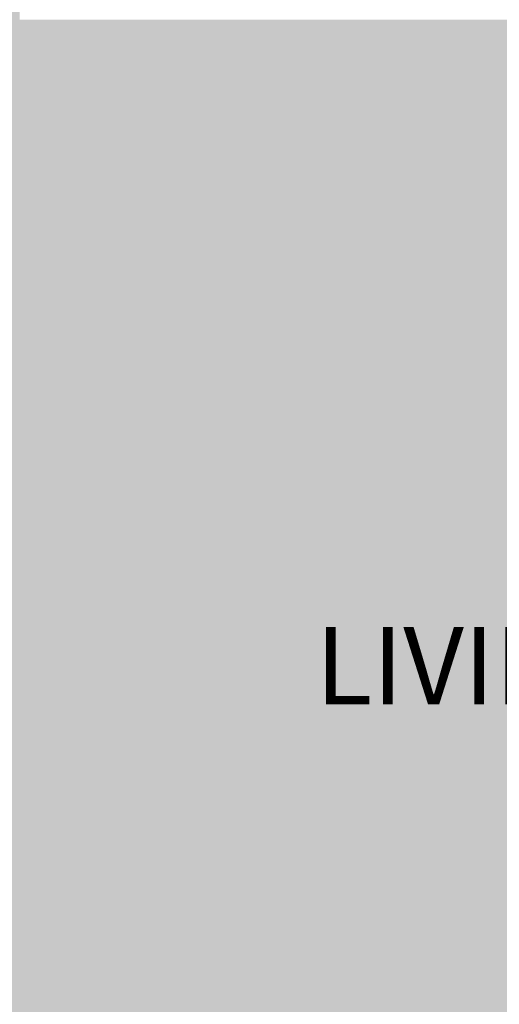
# Model space of a CAD drawing. Units: millimetres. Extents: x -229 to 16545, y -10488 to 4272.
# Tile 13 of 29: x 9556 to 10978, y -4126 to -1208. Entities that reach past the tile are written whole.
import ezdxf

# ---------------------------------------------------------------- set-up
doc = ezdxf.new("R2010")
doc.units = ezdxf.units.MM
doc.layers.add('A-ANNO-DIMS', color=2, linetype='Continuous', lineweight=18)
doc.layers.add('A-AREA-IDEN', color=7, linetype='Continuous', lineweight=18)
doc.layers.add('A-FLOR-PATT', color=254, linetype='Continuous', lineweight=13, true_color=0xfeeab9)
doc.styles.get("Standard").update_dxf_attribs({"font": 'arial.ttf'})
doc.dimstyles.get("Standard").update_dxf_attribs({"dimtxt": 0.18, "dimasz": 0.18, "dimexe": 0.18, "dimexo": 0.0625, "dimgap": 0.09, "dimtad": 0, "dimtih": 1, "dimtoh": 1, "dimdec": 4, "dimzin": 0, "dimdsep": 46, "dimtxsty": 'Standard', "dimcen": 0.09, "dimadec": 0, "dimazin": 0, "dimtfac": 1, "dimtdec": 4, "dimtofl": 0, "dimtmove": 0, "dimatfit": 3, "dimfxl": 1, "dimtolj": 1, "dimtzin": 0, "dimarcsym": 0})

# ---------------------------------------------------------------- blocks, each defined once
blk = doc.blocks.new('*D101')
at = {"layer": 'A-ANNO-DIMS', "color": 0, "lineweight": -2, "transparency": 16777216}
for p, q in [((10907.8, -3049.7), (10908, -3049.7)), ((10907.9, -3049.8), (10907.9, -3049.6)), ((15176.9, -3049.7), (13576.2, -3049.7))]:
    blk.add_line(p, q, dxfattribs=at)
at = {"layer": 'A-ANNO-DIMS', "color": 0, "transparency": 16777216}
blk.add_solid([(13576.2, -3049.7), (13576.2, -3049.7), (13576, -3049.7)], dxfattribs=at)
at = {"layer": 'Defpoints', "color": 0, "transparency": 16777216}
for p in [(10907.9, -3049.7), (13576, -3049.7)]:
    blk.add_point(p, dxfattribs=at)
at = {"layer": 'A-ANNO-DIMS', "color": 0, "transparency": 16777216, "insert": (15177.3, -3049.7), "char_height": 0.18, "attachment_point": 5}
blk.add_mtext('\\A1;R2668', dxfattribs=at)

msp = doc.modelspace()

# ---------------------------------------------------------------- hatches: boundary and pattern name
at = {"layer": 'A-FLOR-PATT', "transparency": 33554592}
h = msp.add_hatch(color=256, dxfattribs=at)
h.dxf.hatch_style = 1
h.paths.add_polyline_path([(7975.933, -5325.772), (7943.121, -5325.772), (7943.121, -4576.49, 0.40145271), (7225.933, -5325.772, 0.40145271), (6508.746, -4576.49), (6508.746, -5325.772), (6475.933, -5325.772), (6475.933, -5438.272), (5975.933, -5438.272), (5975.933, -7267.724), (5975.933, -7438.272), (6478.619, -7438.272), (6463.448, -7355.919), (6464.88, -7356.837), (6463.849, -7358.097), (6478.619, -7438.272), (6610.327, -7438.272), (6632.656, -7409.564), (6632.525, -7406.967), (6634.208, -7407.569), (6619.273, -7426.77), (6654.466, -7438.272), (7610.517, -7438.272), (7607.41, -7421.409), (7608.842, -7422.327), (7607.812, -7423.587), (7610.517, -7438.272), (7975.933, -7438.272)])
h.paths.add_polyline_path([(13785.933, -1208.272), (9555.933, -1208.272), (9555.933, -961.785), (9705.933, -961.785), (9705.933, -918.035), (10704.976, -918.035, 0.40145271), (9705.933, 38.215), (9555.933, 38.215), (9555.933, 2021.728), (5975.933, 2021.728), (5975.933, 755.492), (5745.933, 755.492), (5745.933, 1427.266), (2918.813, 1427.266), (2918.813, -492.942), (5013.319, -492.942), (5013.319, -978.272), (5745.933, -978.272), (5745.933, -397.513), (5975.933, -397.513), (5975.933, -1208.272), (4560.933, -1208.272), (4560.933, -1265.772), (4448.433, -1265.772), (4448.433, -1298.585), (4445.933, -1298.585), (3699.151, -1298.585, 0.40145271), (4448.433, -2015.772), (4560.933, -2015.772), (4560.933, -2384.177), (5745.933, -2384.177), (5799.402, -2384.177), (5799.402, -4518.272), (5975.933, -4518.272), (5975.933, -5208.272), (6475.933, -5208.272), (6475.933, -4575.772), (6508.746, -4575.772), (6508.746, -4576.49, -0.35647263), (7216.672, -5208.272), (7235.194, -5208.272, -0.35647263), (7943.121, -4576.49), (7943.121, -4575.772), (7975.933, -4575.772), (7975.933, -5208.272), (11176.247, -5208.272), (11159.44, -5191.465), (10520.768, -5191.465), (10520.768, -4888.936), (10571.19, -4888.936), (10571.19, -4872.129), (10772.876, -4872.129), (10772.876, -4888.936), (10789.683, -4888.936), (10789.683, -4872.129), (10991.368, -4872.129), (10991.368, -4888.936), (11041.79, -4888.936), (11041.79, -4872.129), (11058.597, -4872.129, -0.09090909), (11428.354, -4872.129), (11445.162, -4872.129), (11445.162, -4888.936), (11529.197, -4888.936), (11529.197, -5191.465), (11327.512, -5191.465), (11310.704, -5208.272), (13785.933, -5208.272)])
h.paths.add_polyline_path([(11047.216, -1630.944, -1), (11402.816, -1630.944, -1)], flags=16)
h.paths.add_polyline_path([(11148.816, -1630.944), (11225.016, -1554.744), (11301.216, -1630.944), (11225.016, -1707.144)], flags=0)
h.paths.add_polyline_path([(11199.616, -1630.944, -1), (11250.416, -1630.944, -1)], flags=0)
h.paths.add_polyline_path([(11588.751, -2096.259), (11588.751, -1543.254, -0.26666697), (12864.918, -1543.254), (12864.918, -2096.259), (12737.302, -2096.259), (12737.302, -2063.121), (11716.368, -2063.121), (11716.368, -2096.259)], flags=16)
h.paths.add_polyline_path([(12012.696, -2489.42), (12600.997, -2489.42), (12600.997, -3666.022), (12012.696, -3666.022)], flags=16)
h.paths.add_polyline_path([(12176.41, -3599.403), (12174.938, -3609.076), (12173.789, -3618.819), (12173.09, -3628.559), (12172.973, -3638.221), (12173.89, -3652.852), (12175.008, -3657.025), (12172.909, -3643.473), (12173.142, -3624.297), (12175.386, -3605.273)], flags=0)
h.paths.add_polyline_path([(8026.289, -286.944), (7737.703, -287.19), (7734.87, -269.156), (8029.092, -268.905)], flags=16)
h.paths.add_polyline_path([(7733.453, -260.139), (7710.784, -115.865), (7557.191, -115.996), (7556.999, 109.744), (7412.687, 132.166), (7412.433, 429.206), (7556.707, 451.876), (7556.568, 614.769), (7412.256, 637.19), (7412.003, 934.231), (7556.276, 956.9), (7556.084, 1182.639), (7709.677, 1182.77), (7732.099, 1327.082), (8029.14, 1327.335), (8051.808, 1183.062), (8205.401, 1183.192), (8205.594, 957.454), (8349.906, 935.031), (8350.159, 637.99), (8205.885, 615.322), (8206.024, 452.43), (8350.336, 430.006), (8350.59, 132.965), (8206.316, 110.298), (8206.509, -115.442), (8052.916, -115.573), (8030.493, -259.885)], flags=16)
h.paths.add_polyline_path([(12261.416, -3475.554), (12262.632, -3486.776), (12264.032, -3497.007), (12265.554, -3506.365), (12267.136, -3514.968), (12268.719, -3522.935), (12271.304, -3535.59), (12273.606, -3548.078), (12275.271, -3561.064), (12275.93, -3574.938), (12275.325, -3590.3), (12273.425, -3607.964), (12270.795, -3625.658), (12268.066, -3641.063), (12266.318, -3649.679), (12265.456, -3653.626), (12263.984, -3659.846), (12264.032, -3659.566), (12264.342, -3658.241), (12264.807, -3656.37), (12265.456, -3653.626), (12266.318, -3649.679), (12267.409, -3644.302), (12268.668, -3637.664), (12270.019, -3630.037), (12271.384, -3621.695), (12272.69, -3612.908), (12273.857, -3603.948), (12274.81, -3595.088), (12275.47, -3586.601), (12275.782, -3578.689), (12275.757, -3571.292), (12275.423, -3564.275), (12274.816, -3557.512), (12273.964, -3550.872), (12272.896, -3544.224), (12271.645, -3537.439), (12270.24, -3530.385), (12267.543, -3517.181), (12264.612, -3501.247), (12261.849, -3481.059)], flags=0)
h.paths.add_polyline_path([(12332.136, -3408.03), (12333.483, -3416.79), (12335.077, -3424.54), (12336.915, -3431.355), (12338.991, -3437.32), (12341.266, -3442.55), (12343.694, -3447.166), (12346.229, -3451.292), (12348.826, -3455.051), (12351.438, -3458.563), (12357.476, -3466.491), (12363.61, -3476.575), (12368.309, -3489.762), (12369.929, -3503.427), (12369.842, -3516.511), (12368.43, -3530.867), (12365.816, -3545.835), (12362.382, -3559.786), (12360.968, -3564.487), (12363.063, -3557.021), (12364.898, -3549.566), (12366.473, -3542.077), (12367.773, -3534.631), (12368.781, -3527.301), (12369.483, -3520.162), (12369.863, -3513.291), (12369.906, -3506.759), (12369.599, -3500.643), (12368.93, -3494.999), (12367.924, -3489.796), (12366.61, -3484.994), (12365.024, -3480.542), (12363.19, -3476.399), (12361.141, -3472.516), (12358.909, -3468.847), (12356.525, -3465.347), (12354.02, -3461.954), (12351.438, -3458.563), (12345.462, -3450.529), (12339.923, -3439.996), (12335.85, -3428.296), (12332.68, -3412.888)], flags=0)
h.paths.add_polyline_path([(12385.287, -3334.612), (12384.977, -3342.409), (12385.02, -3349.196), (12385.4, -3355.066), (12386.104, -3360.105), (12387.112, -3364.41), (12388.412, -3368.071), (12389.987, -3371.181), (12391.823, -3373.832), (12393.919, -3376.097), (12396.337, -3377.978), (12399.153, -3379.462), (12402.445, -3380.531), (12406.289, -3381.172), (12410.758, -3381.371), (12415.935, -3381.106), (12421.893, -3380.368), (12428.658, -3379.159), (12436.069, -3377.55), (12443.907, -3375.635), (12451.961, -3373.505), (12460.015, -3371.254), (12467.853, -3368.971), (12475.263, -3366.749), (12482.029, -3364.68), (12491.877, -3361.657), (12497.701, -3360.107), (12501.639, -3359.288), (12510.135, -3358.326), (12519.662, -3365.412), (12524.243, -3378.911), (12523.764, -3390.7), (12520.746, -3401.577), (12514.248, -3415.634), (12511.518, -3420.418), (12515.856, -3412.154), (12519.153, -3405.024), (12521.516, -3398.804), (12523.049, -3393.276), (12523.865, -3388.212), (12524.059, -3383.441), (12523.7, -3378.958), (12522.853, -3374.815), (12521.576, -3371.054), (12519.931, -3367.722), (12517.982, -3364.865), (12515.786, -3362.529), (12513.405, -3360.758), (12510.877, -3359.588), (12508.136, -3358.982), (12505.086, -3358.897), (12501.639, -3359.288), (12497.701, -3360.107), (12493.183, -3361.309), (12487.988, -3362.851), (12476.403, -3366.408), (12463.335, -3370.326), (12447.372, -3374.788), (12431.759, -3378.604), (12418.504, -3380.974), (12405.811, -3381.624), (12394.725, -3378.025), (12388.039, -3368.367), (12385.583, -3357.877), (12384.826, -3346.204), (12385.428, -3331.059), (12385.953, -3325.719)], flags=0)
h.paths.add_polyline_path([(7880.016, 1173.969), (7880.373, 1175.495), (7880.433, 1175.851), (7879.484, 1171.818)], flags=0)
h.paths.add_polyline_path([(7802.33, 874.962), (7800.771, 885.032), (7798.932, 893.941), (7796.811, 901.774), (7794.419, 908.63), (7791.798, 914.639), (7789.002, 919.945), (7786.083, 924.686), (7783.093, 929.005), (7780.087, 933.043), (7774.996, 939.717), (7768.406, 949.37), (7762.174, 963.427), (7759.342, 978.002), (7758.629, 991.888), (7759.492, 1007.928), (7761.801, 1025.496), (7765.392, 1044.035), (7766.625, 1049.048), (7764.522, 1039.543), (7762.719, 1030.232), (7761.232, 1021.168), (7760.08, 1012.405), (7759.28, 1003.994), (7758.849, 995.988), (7758.806, 988.44), (7759.167, 981.404), (7759.942, 974.914), (7761.104, 968.936), (7762.617, 963.414), (7764.448, 958.299), (7766.559, 953.535), (7768.918, 949.073), (7771.487, 944.856), (7774.232, 940.835), (7777.115, 936.938), (7782.377, 930.041), (7787.845, 922.139), (7793.348, 911.698), (7798.042, 898.247), (7801.702, 880.527)], flags=0)
h.paths.add_polyline_path([(12519.068, -3228.534), (12519.615, -3236.235), (12520.529, -3242.343), (12521.78, -3247.103), (12523.337, -3250.758), (12525.171, -3253.556), (12527.248, -3255.709), (12529.522, -3257.296), (12531.95, -3258.361), (12534.486, -3258.949), (12537.082, -3259.11), (12539.694, -3258.888), (12542.277, -3258.329), (12544.781, -3257.478), (12547.173, -3256.388), (12549.46, -3255.129), (12550.455, -3254.517), (12555.825, -3251.109), (12557.835, -3249.942), (12565.181, -3246.404), (12574.565, -3253.032), (12576.931, -3265.022), (12576.627, -3277.425), (12575.416, -3290.819), (12574.851, -3295.392), (12575.708, -3287.593), (12576.322, -3280.806), (12576.688, -3274.939), (12576.812, -3269.899), (12576.688, -3265.593), (12576.322, -3261.932), (12575.708, -3258.822), (12574.851, -3256.172), (12573.753, -3253.905), (12572.439, -3252.005), (12570.943, -3250.474), (12569.293, -3249.309), (12567.523, -3248.513), (12565.658, -3248.083), (12563.732, -3248.022), (12561.777, -3248.328), (12559.814, -3248.989), (12557.835, -3249.942), (12555.825, -3251.109), (12553.77, -3252.413), (12551.652, -3253.78), (12549.46, -3255.129), (12543.167, -3258.594), (12532.661, -3259.485), (12524.685, -3253.923), (12520.949, -3245.152), (12519.138, -3233.042)], flags=0)
h.paths.add_polyline_path([(7741.293, 790.501), (7741.641, 799.467), (7741.584, 807.269), (7741.141, 814.015), (7740.329, 819.809), (7739.165, 824.757), (7737.667, 828.966), (7735.853, 832.541), (7733.74, 835.586), (7731.348, 838.188), (7728.71, 840.348), (7725.861, 842.052), (7722.836, 843.28), (7719.671, 844.015), (7716.4, 844.237), (7713.06, 843.932), (7709.684, 843.081), (7706.304, 841.686), (7702.923, 839.834), (7699.543, 837.629), (7696.164, 835.178), (7692.784, 832.585), (7684.718, 826.315), (7675.609, 820.63), (7664.001, 817.274), (7654.105, 821.884), (7647.171, 832.02), (7644.191, 846.522), (7646.321, 860.288), (7647.49, 864.223), (7645.946, 857.865), (7645.046, 852.044), (7644.827, 846.557), (7645.243, 841.404), (7646.221, 836.642), (7647.693, 832.318), (7649.587, 828.489), (7651.832, 825.206), (7654.359, 822.523), (7657.097, 820.49), (7659.984, 819.145), (7662.993, 818.452), (7666.108, 818.357), (7669.311, 818.809), (7672.583, 819.755), (7675.908, 821.139), (7679.268, 822.913), (7682.645, 825.021), (7686.025, 827.401), (7689.404, 829.958), (7692.784, 832.585), (7700.505, 838.509), (7709.871, 843.64), (7721.436, 844.698), (7733.277, 837.617), (7739.571, 825.214), (7741.557, 811.049), (7741.669, 795.575)], flags=0)
h.paths.add_polyline_path([(8377.641, 137.216), (8359.607, 134.382), (8359.356, 428.605), (8377.395, 425.802)], flags=16)
h.paths.add_polyline_path([(7650.715, 668.465), (7650.08, 677.319), (7649.023, 684.34), (7647.579, 689.811), (7645.785, 694.012), (7643.675, 697.228), (7641.286, 699.7), (7638.669, 701.521), (7635.876, 702.744), (7632.96, 703.419), (7629.974, 703.601), (7626.971, 703.344), (7624.004, 702.697), (7621.125, 701.717), (7618.375, 700.462), (7615.749, 699.013), (7614.561, 698.279), (7608.435, 694.382), (7606.125, 693.04), (7598.981, 689.594), (7589.669, 693.773), (7585.26, 702.856), (7584.221, 713.11), (7584.49, 724.584), (7585.863, 739.937), (7586.518, 745.277), (7585.539, 736.31), (7584.841, 728.507), (7584.424, 721.761), (7584.288, 715.966), (7584.433, 711.016), (7584.86, 706.807), (7585.567, 703.231), (7586.556, 700.186), (7587.821, 697.58), (7589.332, 695.397), (7591.053, 693.637), (7592.951, 692.3), (7594.989, 691.385), (7597.132, 690.895), (7599.346, 690.826), (7601.594, 691.18), (7603.851, 691.943), (7606.125, 693.04), (7608.435, 694.382), (7610.797, 695.885), (7613.229, 697.458), (7620.475, 701.929), (7632.001, 704.44), (7643.476, 699.417), (7648.536, 687.571), (7650.63, 673.661)], flags=0)
h.paths.add_polyline_path([(7385.628, 136.37), (7385.382, 424.956), (7403.416, 427.789), (7403.667, 133.567)], flags=16)
h.paths.add_polyline_path([(12993.884, -2257.186), (12959.588, -2257.186), (12959.588, -2125.099), (13531.966, -2125.099, -0.19047621), (13531.966, -3974.321), (12959.588, -3974.321), (12959.588, -3842.233), (12993.884, -3842.233)], flags=16)
h.paths.add_polyline_path([(13413.486, -3313.884), (13413.486, -2785.535), (13562.885, -2785.535, -0.04962821), (13562.885, -3313.884)], flags=0)
h.paths.add_polyline_path([(8377.21, 642.241), (8359.176, 639.407), (8358.925, 933.629), (8376.964, 930.826)], flags=16)
h.paths.add_polyline_path([(13086.058, -1864.83), (13086.058, -1449.84), (13501.048, -1449.84), (13501.048, -1864.83)], flags=16)
h.paths.add_polyline_path([(13305.814, -1862.197), (13302.103, -1859.624), (13298.088, -1857.068), (13293.799, -1854.536), (13289.262, -1852.031), (13284.504, -1849.559), (13279.554, -1847.125), (13274.439, -1844.735), (13269.17, -1842.389), (13263.701, -1840.081), (13257.97, -1837.797), (13251.914, -1835.525), (13245.472, -1833.252), (13238.582, -1830.968), (13231.18, -1828.66), (13223.206, -1826.315), (13209.182, -1822.458), (13204.584, -1821.48), (13217.962, -1824.773), (13235.072, -1829.804), (13248.777, -1834.349), (13260.829, -1838.869), (13274.479, -1844.63), (13289.675, -1852.101), (13302.553, -1859.704)], flags=0)
h.paths.add_polyline_path([(13428.104, -1820.994), (13419.007, -1818.141), (13409.95, -1815.4), (13400.766, -1812.747), (13391.271, -1810.151), (13376.087, -1806.251), (13370.618, -1805.019), (13386.304, -1808.794), (13405.087, -1813.928), (13423.014, -1819.354)], flags=0)
h.paths.add_polyline_path([(7385.197, 641.395), (7384.951, 929.98), (7402.986, 932.814), (7403.236, 638.592)], flags=16)
h.paths.add_polyline_path([(13262.537, -1725.526), (13253.246, -1724.74), (13244.516, -1724.117), (13235.94, -1723.625), (13223.267, -1723.062), (13217.598, -1722.912), (13231.966, -1723.397), (13248.733, -1724.359), (13266.899, -1725.895), (13272.802, -1726.502)], flags=0)
h.paths.add_polyline_path([(13191.893, -1641.137), (13208.675, -1640.506), (13214.057, -1640.258), (13197.763, -1640.936)], flags=0)
h.paths.add_polyline_path([(13097.524, -1608.457), (13114.284, -1609.031), (13120.126, -1609.105), (13103.045, -1608.71)], flags=0)
h.paths.add_polyline_path([(13465.328, -1521.577), (13473.906, -1517.015), (13481.761, -1511.636), (13492.562, -1502.076), (13495.327, -1497.933), (13485.818, -1508.858), (13470.208, -1519.547)], flags=0)
h.paths.add_polyline_path([(13175.015, -1500.891), (13184.046, -1501.807), (13192.721, -1502.52), (13201.114, -1503.034), (13209.273, -1503.351), (13217.244, -1503.476), (13225.078, -1503.41), (13232.821, -1503.16), (13240.524, -1502.728), (13248.233, -1502.117), (13255.993, -1501.322), (13263.825, -1500.293), (13271.746, -1498.974), (13279.775, -1497.305), (13287.928, -1495.229), (13296.222, -1492.688), (13304.675, -1489.622), (13313.304, -1485.975), (13322.089, -1481.727), (13330.859, -1477.028), (13339.408, -1472.063), (13347.526, -1467.02), (13355.006, -1462.087), (13364.86, -1455.202), (13367.224, -1453.299), (13358.544, -1459.754), (13343.348, -1469.775), (13326.143, -1479.767), (13309.023, -1488.045), (13292.249, -1494.129), (13276.009, -1498.264), (13260.299, -1500.88), (13244.401, -1502.51), (13228.945, -1503.378), (13213.316, -1503.508), (13197.047, -1502.876), (13180.088, -1501.481)], flags=0)
h.paths.add_polyline_path([(7733.501, 1336.101), (7736.303, 1354.14), (8024.889, 1354.386), (8027.723, 1336.352)], flags=16)

# ---------------------------------------------------------------- texts
at = {"layer": 'A-AREA-IDEN'}
msp.add_text('LIVING', height=228.5841, dxfattribs=at).set_placement((10432.603, -3236.78))

# ---------------------------------------------------------------- dimensions: what is measured, and where the dimension line sits
at = {"layer": 'A-ANNO-DIMS'}
dim = msp.add_radius_dim(center=(10907.903, -3049.71), mpoint=(13575.995, -3049.709), dimstyle='Standard', override={"dimdec": 0, "dimlfac": 1, "dimrnd": 0, "dimzin": 0, "dimdsep": 46, "dimlunit": 2}, dxfattribs=at)
dim.commit()
dim.dimension.update_dxf_attribs({"geometry": '*D101', "text_midpoint": (15176.85, -3049.708), "dimtype": 164})

doc.saveas('drawing.dxf')
